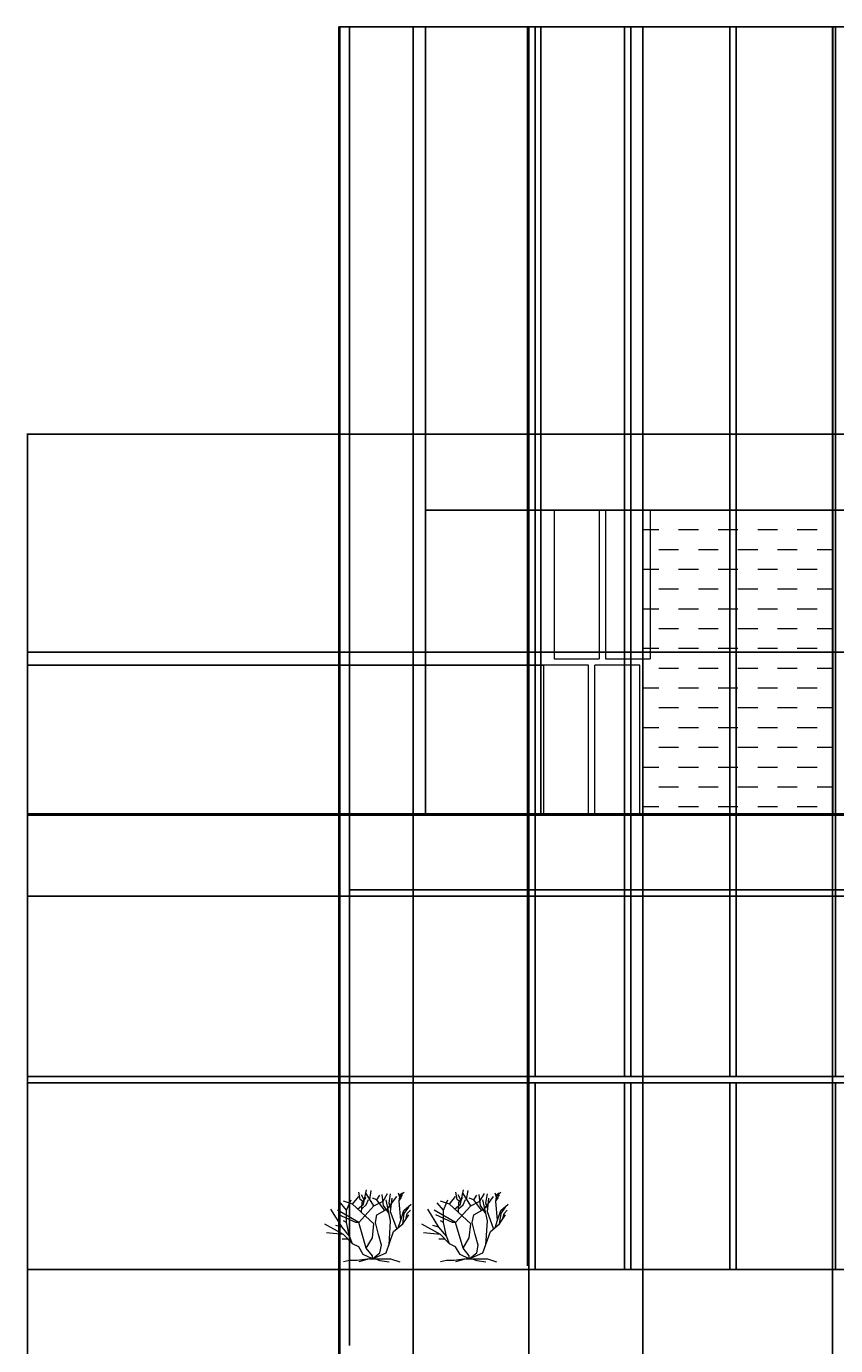
# Model space of a CAD drawing. Units: inches. Extents: x 250 to 1217, y -42 to 832.
# Tile 3 of 7: x 250 to 506, y 415 to 832. Entities that reach past the tile are written whole.
import ezdxf

# ---------------------------------------------------------------- set-up
doc = ezdxf.new("R2010")
doc.units = ezdxf.units.IN
doc.header["$MEASUREMENT"] = 0
for name, color, linetype, lineweight in [('A-ANNO-DIMS', 2, 'Continuous', 18), ('A-ELEV', 7, 'Continuous', 25), ('A-ELEV-PATT', 8, 'Continuous', 13), ('A-GLAZ', 4, 'Continuous', 18), ('L-PLNT', 3, 'Continuous', 13)]:
    doc.layers.add(name, color=color, linetype=linetype, lineweight=lineweight)
doc.styles.get("Standard").update_dxf_attribs({"font": 'arial.ttf'})
doc.dimstyles.get("Standard").update_dxf_attribs({"dimtxt": 0.18, "dimasz": 0.18, "dimexe": 0.18, "dimexo": 0.0625, "dimgap": 0.09, "dimtad": 0, "dimtih": 1, "dimtoh": 1, "dimdec": 4, "dimzin": 0, "dimdsep": 46, "dimtxsty": 'Standard', "dimcen": 0.09, "dimadec": 0, "dimazin": 0, "dimtfac": 1, "dimtdec": 4, "dimtofl": 0, "dimtmove": 0, "dimatfit": 3, "dimfxl": 1, "dimtolj": 1, "dimtzin": 0, "dimarcsym": 0})

# ---------------------------------------------------------------- blocks, each defined once
blk = doc.blocks.new('*U2')
for p, q in [((-12.471, 19.775), (-12.898, 22.044)), ((-11.28, 19.619), (-12.104, 21.184)), ((-11.433, 18.289), (-10.457, 22.749)), ((-8.16, 17.76), (-10.56, 21.6)), ((-9.48, 19.775), (-8.992, 22.592)), ((-7.2, 19.68), (-6.24, 21.12)), ((-5.086, 17.741), (-5.513, 21.34)), ((-5.28, 19.2), (-3.84, 21.6)), ((-3.377, 18.602), (-2.888, 21.575)), ((-0.508, 21.888), (-0.081, 20.558)), ((-0.203, 19.149), (0.102, 21.34)), ((-0.02, 20.01), (0.896, 21.105)), ((0.041, 20.714), (1.384, 22.044)), ((0.102, 21.34), (0.835, 21.888)), ((-16.8, 16.32), (-18.72, 18.72)), ((-14.88, 18.24), (-17.76, 19.2)), ((-16.8, 16.32), (-15.36, 19.68)), ((-14.88, 18.24), (-12.96, 20.64)), ((-8.16, 12), (-14.88, 18.24)), ((-13.325, 16.724), (-11.433, 18.289)), ((-12.96, 12.48), (-8.16, 17.76)), ((-11.677, 19.071), (-12.471, 19.775)), ((-12.043, 15.628), (-11.921, 18.836)), ((-11.982, 16.802), (-10.579, 18.054)), ((-11.921, 18.836), (-10.64, 20.401)), ((-10.579, 18.054), (-9.846, 19.697)), ((-7.2, 19.68), (-8.64, 20.16)), ((-8.16, 17.76), (-5.28, 19.2)), ((-4.8, 16.32), (-7.2, 19.68)), ((-7.2, 14.88), (-3.84, 16.8)), ((-3.377, 15.315), (-5.086, 17.819)), ((-2.88, 12.96), (-4.32, 19.68)), ((-3.84, 16.8), (-0.96, 20.64)), ((-2.766, 16.802), (-3.377, 18.602)), ((-2.88, 15.84), (-2.4, 20.16)), ((0.346, 13.203), (-0.203, 19.149)), ((-0.142, 19.384), (0.59, 20.401)), ((1.323, 16.254), (3.642, 18.289)), ((1.44, 15.36), (2.88, 17.28)), ((-18.24, 11.04), (-21.755, 16.655)), ((-12.96, 12.48), (-19.68, 16.32)), ((-13.92, 12.48), (-19.2, 14.88)), ((-16.8, 12.48), (-17.76, 12.96)), ((-16.8, 12.48), (-16.8, 16.32)), ((-7.68, 12.48), (-7.2, 14.88)), ((-3.36, 5.28), (-2.88, 12.96)), ((-0.96, 10.56), (-2.88, 15.84)), ((-0.48, 10.8), (0.346, 13.203)), ((0.346, 13.203), (1.323, 16.254)), ((0.96, 12), (1.44, 15.36)), ((0.96, 12), (2.88, 14.88)), ((1.92, 13.44), (2.4, 15.36)), ((2.4, 15.36), (3.36, 16.32)), ((-17.76, 8.64), (-23.663, 11.961)), ((-17.76, 8.64), (-23.128, 9.222)), ((-18.24, 11.04), (-20.16, 11.52)), ((-15.84, 8.16), (-18.24, 11.04)), ((-14.88, 5.76), (-17.76, 8.64)), ((-15.84, 8.16), (-16.8, 12.48)), ((-12.96, 12.48), (-13.92, 12.48)), ((-10.56, 4.32), (-12.96, 12.48)), ((-8.64, 7.68), (-8.16, 12)), ((-6.72, 8.64), (-7.68, 12.48)), ((-5.76, 5.28), (-6.72, 8.64)), ((-4.32, 2.88), (-1.92, 9.6)), ((-1.92, 9.6), (0.96, 12)), ((-16.32, 7.2), (-18.24, 7.2)), ((-14.88, 5.76), (-15.84, 8.16)), ((-12.96, 4.8), (-14.88, 5.76)), ((-11.52, 2.4), (-12.96, 4.8)), ((-10.56, 4.32), (-8.64, 7.68)), ((-8.64, 1.92), (-10.56, 4.32)), ((-6.24, 2.88), (-5.76, 5.28)), ((-15.84, 0.48), (-17.76, 0)), ((-13.44, 0.48), (-15.84, 0.48)), ((-9.6, 0.96), (-13.44, 0.48)), ((-9.6, 0.96), (-12.96, 0)), ((-8.64, 0.96), (-11.52, 2.4)), ((-9.6, 0.96), (-7.68, 0.96)), ((-8.64, 0.96), (-4.32, 2.88)), ((-8.64, 0.96), (-6.24, 2.88)), ((-8.64, 0.96), (-8.64, 1.92)), ((-8.64, 0.96), (-2.88, 0.96)), ((-7.68, 0.96), (-6.24, 0.48)), ((-6.24, 0.48), (-3.36, 0)), ((-2.88, 0.96), (0, 0))]:
    blk.add_line(p, q)
blk = doc.blocks.new('WIN-PANEL-NARROW')
for p, q in [((0, 47), (0, 0)), ((14.16, 47), (14.16, 0)), ((0, 0), (14.16, 0))]:
    blk.add_line(p, q)
blk = doc.blocks.new('*D8')
at = {"layer": 'A-ANNO-DIMS', "color": 0, "lineweight": -2, "transparency": 16777216}
for p, q in [((352.34, 702.99), (352.34, 831.77)), ((352.52, 831.59), (491.1, 831.59)), ((630.6, 831.59), (492.03, 831.59)), ((630.78, 702.99), (630.78, 831.77))]:
    blk.add_line(p, q, dxfattribs=at)
at = {"layer": 'A-ANNO-DIMS', "color": 0, "transparency": 16777216}
for points in [[(352.52, 831.62), (352.52, 831.56), (352.34, 831.59)], [(630.6, 831.62), (630.6, 831.56), (630.78, 831.59)]]:
    blk.add_solid(points, dxfattribs=at)
at = {"layer": 'Defpoints', "color": 0, "transparency": 16777216}
for p in [(630.78, 831.59), (352.34, 702.93), (630.78, 702.93)]:
    blk.add_point(p, dxfattribs=at)
at = {"layer": 'A-ANNO-DIMS', "color": 0, "transparency": 16777216, "insert": (491.56, 831.59), "char_height": 0.18, "attachment_point": 5}
blk.add_mtext('\\A1;278.44', dxfattribs=at)
blk = doc.blocks.new('*D11')
at = {"layer": 'A-ANNO-DIMS', "color": 0, "lineweight": -2, "transparency": 16777216}
for p, q in [((352.28, 702.93), (250.36, 702.93)), ((250.54, 702.75), (250.54, 390.68)), ((250.54, 78.24), (250.54, 390.31)), ((347.84, 78.06), (250.36, 78.06))]:
    blk.add_line(p, q, dxfattribs=at)
at = {"layer": 'A-ANNO-DIMS', "color": 0, "transparency": 16777216}
for points in [[(250.51, 702.75), (250.57, 702.75), (250.54, 702.93)], [(250.51, 78.24), (250.57, 78.24), (250.54, 78.06)]]:
    blk.add_solid(points, dxfattribs=at)
at = {"layer": 'Defpoints', "color": 0, "transparency": 16777216}
for p in [(250.54, 702.93), (352.34, 702.93), (347.9, 78.06)]:
    blk.add_point(p, dxfattribs=at)
at = {"layer": 'A-ANNO-DIMS', "color": 0, "transparency": 16777216, "insert": (250.54, 390.49), "char_height": 0.18, "attachment_point": 5}
blk.add_mtext('\\A1;624.9', dxfattribs=at)
blk = doc.blocks.new('*D22')
at = {"layer": 'A-ANNO-DIMS', "color": 0, "lineweight": -2, "transparency": 16777216}
for p, q in [((349.2, 175.91), (349.2, 831.77)), ((349.38, 831.59), (378.7, 831.59)), ((408.8, 831.59), (379.49, 831.59)), ((408.98, 174.99), (408.98, 831.77))]:
    blk.add_line(p, q, dxfattribs=at)
at = {"layer": 'A-ANNO-DIMS', "color": 0, "transparency": 16777216}
for points in [[(349.38, 831.62), (349.38, 831.56), (349.2, 831.59)], [(408.8, 831.62), (408.8, 831.56), (408.98, 831.59)]]:
    blk.add_solid(points, dxfattribs=at)
at = {"layer": 'Defpoints', "color": 0, "transparency": 16777216}
for p in [(408.98, 831.59), (349.2, 175.84), (408.98, 174.93)]:
    blk.add_point(p, dxfattribs=at)
at = {"layer": 'A-ANNO-DIMS', "color": 0, "transparency": 16777216, "insert": (379.09, 831.59), "char_height": 0.18, "attachment_point": 5}
blk.add_mtext('\\A1;59.78', dxfattribs=at)
blk = doc.blocks.new('*D23')
at = {"layer": 'A-ANNO-DIMS', "color": 0, "lineweight": -2, "transparency": 16777216}
for p, q in [((408.98, 174.99), (408.98, 831.77)), ((409.16, 831.59), (426.76, 831.59)), ((444.8, 831.59), (427.2, 831.59)), ((444.98, 174.99), (444.98, 831.77))]:
    blk.add_line(p, q, dxfattribs=at)
at = {"layer": 'A-ANNO-DIMS', "color": 0, "transparency": 16777216}
for points in [[(409.16, 831.62), (409.16, 831.56), (408.98, 831.59)], [(444.8, 831.62), (444.8, 831.56), (444.98, 831.59)]]:
    blk.add_solid(points, dxfattribs=at)
at = {"layer": 'Defpoints', "color": 0, "transparency": 16777216}
for p in [(444.98, 831.59), (408.98, 174.93), (444.98, 174.93)]:
    blk.add_point(p, dxfattribs=at)
at = {"layer": 'A-ANNO-DIMS', "color": 0, "transparency": 16777216, "insert": (426.98, 831.59), "char_height": 0.18, "attachment_point": 5}
blk.add_mtext('\\A1;36', dxfattribs=at)
blk = doc.blocks.new('*D24')
at = {"layer": 'A-ANNO-DIMS', "color": 0, "lineweight": -2, "transparency": 16777216}
for p, q in [((444.98, 174.99), (444.98, 831.77)), ((445.16, 831.59), (474.76, 831.59)), ((504.8, 831.59), (475.2, 831.59)), ((504.98, 174.99), (504.98, 831.77))]:
    blk.add_line(p, q, dxfattribs=at)
at = {"layer": 'A-ANNO-DIMS', "color": 0, "transparency": 16777216}
for points in [[(445.16, 831.62), (445.16, 831.56), (444.98, 831.59)], [(504.8, 831.62), (504.8, 831.56), (504.98, 831.59)]]:
    blk.add_solid(points, dxfattribs=at)
at = {"layer": 'Defpoints', "color": 0, "transparency": 16777216}
for p in [(504.98, 831.59), (444.98, 174.93), (504.98, 174.93)]:
    blk.add_point(p, dxfattribs=at)
at = {"layer": 'A-ANNO-DIMS', "color": 0, "transparency": 16777216, "insert": (474.98, 831.59), "char_height": 0.18, "attachment_point": 5}
blk.add_mtext('\\A1;60', dxfattribs=at)
blk = doc.blocks.new('*D25')
at = {"layer": 'A-ANNO-DIMS', "color": 0, "lineweight": -2, "transparency": 16777216}
for p, q in [((504.98, 174.99), (504.98, 831.77)), ((505.16, 831.59), (522.76, 831.59)), ((540.8, 831.59), (523.2, 831.59)), ((540.98, 174.99), (540.98, 831.77))]:
    blk.add_line(p, q, dxfattribs=at)
at = {"layer": 'A-ANNO-DIMS', "color": 0, "transparency": 16777216}
for points in [[(505.16, 831.62), (505.16, 831.56), (504.98, 831.59)], [(540.8, 831.62), (540.8, 831.56), (540.98, 831.59)]]:
    blk.add_solid(points, dxfattribs=at)
at = {"layer": 'Defpoints', "color": 0, "transparency": 16777216}
for p in [(540.98, 831.59), (504.98, 174.93), (540.98, 174.93)]:
    blk.add_point(p, dxfattribs=at)
at = {"layer": 'A-ANNO-DIMS', "color": 0, "transparency": 16777216, "insert": (522.98, 831.59), "char_height": 0.18, "attachment_point": 5}
blk.add_mtext('\\A1;36', dxfattribs=at)
blk = doc.blocks.new('*D38')
at = {"layer": 'A-ANNO-DIMS', "color": 0, "lineweight": -2, "transparency": 16777216}
for p, q in [((413.675954, 629.927068), (250.356906, 629.927068)), ((250.536906, 629.747068), (250.536906, 606.607068)), ((250.536906, 583.107068), (250.536906, 606.247068)), ((412.675954, 582.927068), (250.356906, 582.927068))]:
    blk.add_line(p, q, dxfattribs=at)
at = {"layer": 'A-ANNO-DIMS', "color": 0, "transparency": 16777216}
for points in [[(250.506906, 629.747068), (250.566906, 629.747068), (250.536906, 629.927068)], [(250.506906, 583.107068), (250.566906, 583.107068), (250.536906, 582.927068)]]:
    blk.add_solid(points, dxfattribs=at)
at = {"layer": 'Defpoints', "color": 0, "transparency": 16777216}
for p in [(250.536906, 629.927068), (413.738454, 629.927068), (412.738454, 582.927068)]:
    blk.add_point(p, dxfattribs=at)
at = {"layer": 'A-ANNO-DIMS', "color": 0, "transparency": 16777216, "insert": (250.536906, 606.427068), "char_height": 0.18, "attachment_point": 5}
blk.add_mtext('\\A1;47', dxfattribs=at)
blk = doc.blocks.new('*D39')
at = {"layer": 'A-ANNO-DIMS', "color": 0, "lineweight": -2, "transparency": 16777216}
for p, q in [((352.34, 558.99), (352.34, 831.77)), ((352.52, 831.59), (364.12, 831.59)), ((376.16, 831.59), (364.56, 831.59)), ((376.34, 582.99), (376.34, 831.77))]:
    blk.add_line(p, q, dxfattribs=at)
at = {"layer": 'A-ANNO-DIMS', "color": 0, "transparency": 16777216}
for points in [[(352.52, 831.62), (352.52, 831.56), (352.34, 831.59)], [(376.16, 831.62), (376.16, 831.56), (376.34, 831.59)]]:
    blk.add_solid(points, dxfattribs=at)
at = {"layer": 'Defpoints', "color": 0, "transparency": 16777216}
for p in [(352.34, 831.59), (376.34, 582.93), (352.34, 558.93)]:
    blk.add_point(p, dxfattribs=at)
at = {"layer": 'A-ANNO-DIMS', "color": 0, "transparency": 16777216, "insert": (364.34, 831.59), "char_height": 0.18, "attachment_point": 5}
blk.add_mtext('\\A1;24', dxfattribs=at)
blk = doc.blocks.new('*D40')
at = {"layer": 'A-ANNO-DIMS', "color": 0, "lineweight": -2, "transparency": 16777216}
for p, q in [((376.34, 678.99), (376.34, 831.77)), ((376.52, 831.59), (394.08, 831.59)), ((412.56, 831.59), (395, 831.59)), ((412.74, 678.99), (412.74, 831.77))]:
    blk.add_line(p, q, dxfattribs=at)
at = {"layer": 'A-ANNO-DIMS', "color": 0, "transparency": 16777216}
for points in [[(376.52, 831.62), (376.52, 831.56), (376.34, 831.59)], [(412.56, 831.62), (412.56, 831.56), (412.74, 831.59)]]:
    blk.add_solid(points, dxfattribs=at)
at = {"layer": 'Defpoints', "color": 0, "transparency": 16777216}
for p in [(412.74, 831.59), (376.34, 678.93), (412.74, 678.93)]:
    blk.add_point(p, dxfattribs=at)
at = {"layer": 'A-ANNO-DIMS', "color": 0, "transparency": 16777216, "insert": (394.54, 831.59), "char_height": 0.18, "attachment_point": 5}
blk.add_mtext('\\A1;36.396', dxfattribs=at)
blk = doc.blocks.new('*D41')
at = {"layer": 'A-ANNO-DIMS', "color": 0, "lineweight": -2, "transparency": 16777216}
for p, q in [((412.74, 678.99), (412.74, 831.77)), ((412.92, 831.59), (428.44, 831.59)), ((444.88, 831.59), (429.37, 831.59)), ((445.06, 678.99), (445.06, 831.77))]:
    blk.add_line(p, q, dxfattribs=at)
at = {"layer": 'A-ANNO-DIMS', "color": 0, "transparency": 16777216}
for points in [[(412.92, 831.62), (412.92, 831.56), (412.74, 831.59)], [(444.88, 831.62), (444.88, 831.56), (445.06, 831.59)]]:
    blk.add_solid(points, dxfattribs=at)
at = {"layer": 'Defpoints', "color": 0, "transparency": 16777216}
for p in [(445.06, 831.59), (412.74, 678.93), (445.06, 678.93)]:
    blk.add_point(p, dxfattribs=at)
at = {"layer": 'A-ANNO-DIMS', "color": 0, "transparency": 16777216, "insert": (428.9, 831.59), "char_height": 0.18, "attachment_point": 5}
blk.add_mtext('\\A1;32.326', dxfattribs=at)
blk = doc.blocks.new('*D42')
at = {"layer": 'A-ANNO-DIMS', "color": 0, "lineweight": -2, "transparency": 16777216}
for p, q in [((445.06, 678.99), (445.06, 831.77)), ((445.24, 831.59), (474.85, 831.59)), ((504.88, 831.59), (475.28, 831.59)), ((505.06, 678.99), (505.06, 831.77))]:
    blk.add_line(p, q, dxfattribs=at)
at = {"layer": 'A-ANNO-DIMS', "color": 0, "transparency": 16777216}
for points in [[(445.24, 831.62), (445.24, 831.56), (445.06, 831.59)], [(504.88, 831.62), (504.88, 831.56), (505.06, 831.59)]]:
    blk.add_solid(points, dxfattribs=at)
at = {"layer": 'Defpoints', "color": 0, "transparency": 16777216}
for p in [(505.06, 831.59), (445.06, 678.93), (505.06, 678.93)]:
    blk.add_point(p, dxfattribs=at)
at = {"layer": 'A-ANNO-DIMS', "color": 0, "transparency": 16777216, "insert": (475.06, 831.59), "char_height": 0.18, "attachment_point": 5}
blk.add_mtext('\\A1;60', dxfattribs=at)
blk = doc.blocks.new('*D43')
at = {"layer": 'A-ANNO-DIMS', "color": 0, "lineweight": -2, "transparency": 16777216}
for p, q in [((505.06, 678.99), (505.06, 831.77)), ((505.24, 831.59), (512.61, 831.59)), ((520.89, 831.59), (513.52, 831.59)), ((521.07, 678.99), (521.07, 831.77))]:
    blk.add_line(p, q, dxfattribs=at)
at = {"layer": 'A-ANNO-DIMS', "color": 0, "transparency": 16777216}
for points in [[(505.24, 831.62), (505.24, 831.56), (505.06, 831.59)], [(520.89, 831.62), (520.89, 831.56), (521.07, 831.59)]]:
    blk.add_solid(points, dxfattribs=at)
at = {"layer": 'Defpoints', "color": 0, "transparency": 16777216}
for p in [(521.07, 831.59), (505.06, 678.93), (521.07, 678.93)]:
    blk.add_point(p, dxfattribs=at)
at = {"layer": 'A-ANNO-DIMS', "color": 0, "transparency": 16777216, "insert": (513.07, 831.59), "char_height": 0.18, "attachment_point": 5}
blk.add_mtext('\\A1;16.002', dxfattribs=at)
blk = doc.blocks.new('*D49')
at = {"layer": 'A-ANNO-DIMS', "color": 0, "lineweight": -2, "transparency": 16777216}
for p, q in [((348.98, 318.99), (348.98, 831.77)), ((349.16, 831.59), (489.48, 831.59)), ((630.6, 831.59), (490.28, 831.59)), ((630.78, 318.99), (630.78, 831.77))]:
    blk.add_line(p, q, dxfattribs=at)
at = {"layer": 'A-ANNO-DIMS', "color": 0, "transparency": 16777216}
for points in [[(349.16, 831.62), (349.16, 831.56), (348.98, 831.59)], [(630.6, 831.62), (630.6, 831.56), (630.78, 831.59)]]:
    blk.add_solid(points, dxfattribs=at)
at = {"layer": 'Defpoints', "color": 0, "transparency": 16777216}
for p in [(630.78, 831.59), (348.98, 318.93), (630.78, 318.93)]:
    blk.add_point(p, dxfattribs=at)
at = {"layer": 'A-ANNO-DIMS', "color": 0, "transparency": 16777216, "insert": (489.88, 831.59), "char_height": 0.18, "attachment_point": 5}
blk.add_mtext('\\A1;281.8', dxfattribs=at)
blk = doc.blocks.new('*D51')
at = {"layer": 'A-ANNO-DIMS', "color": 0, "lineweight": -2, "transparency": 16777216}
for p, q in [((348.98, 198.99), (348.98, 831.77)), ((349.16, 831.59), (360.27, 831.59)), ((372.3, 831.59), (361.2, 831.59)), ((372.48, 199.88), (372.48, 831.77))]:
    blk.add_line(p, q, dxfattribs=at)
at = {"layer": 'A-ANNO-DIMS', "color": 0, "transparency": 16777216}
for points in [[(349.16, 831.62), (349.16, 831.56), (348.98, 831.59)], [(372.3, 831.62), (372.3, 831.56), (372.48, 831.59)]]:
    blk.add_solid(points, dxfattribs=at)
at = {"layer": 'Defpoints', "color": 0, "transparency": 16777216}
for p in [(372.48, 831.59), (348.98, 198.93), (372.48, 199.81)]:
    blk.add_point(p, dxfattribs=at)
at = {"layer": 'A-ANNO-DIMS', "color": 0, "transparency": 16777216, "insert": (360.73, 831.59), "char_height": 0.18, "attachment_point": 5}
blk.add_mtext('\\A1;23.496', dxfattribs=at)
blk = doc.blocks.new('*D53')
at = {"layer": 'A-ANNO-DIMS', "color": 0, "lineweight": -2, "transparency": 16777216}
for p, q in [((352.34, 438.99), (352.34, 831.77)), ((352.52, 831.59), (380.04, 831.59)), ((408.34, 831.59), (380.83, 831.59)), ((408.52, 440.1), (408.52, 831.77))]:
    blk.add_line(p, q, dxfattribs=at)
at = {"layer": 'A-ANNO-DIMS', "color": 0, "transparency": 16777216}
for points in [[(352.52, 831.62), (352.52, 831.56), (352.34, 831.59)], [(408.34, 831.62), (408.34, 831.56), (408.52, 831.59)]]:
    blk.add_solid(points, dxfattribs=at)
at = {"layer": 'Defpoints', "color": 0, "transparency": 16777216}
for p in [(408.52, 831.59), (352.34, 438.93), (408.52, 440.03)]:
    blk.add_point(p, dxfattribs=at)
at = {"layer": 'A-ANNO-DIMS', "color": 0, "transparency": 16777216, "insert": (380.43, 831.59), "char_height": 0.18, "attachment_point": 5}
blk.add_mtext('\\A1;56.18', dxfattribs=at)
blk = doc.blocks.new('*D54')
at = {"layer": 'A-ANNO-DIMS', "color": 0, "lineweight": -2, "transparency": 16777216}
for p, q in [((408.52, 440.1), (408.52, 831.77)), ((408.7, 831.59), (474.4, 831.59)), ((541, 831.59), (475.31, 831.59)), ((541.18, 438.99), (541.18, 831.77))]:
    blk.add_line(p, q, dxfattribs=at)
at = {"layer": 'A-ANNO-DIMS', "color": 0, "transparency": 16777216}
for points in [[(408.7, 831.62), (408.7, 831.56), (408.52, 831.59)], [(541, 831.62), (541, 831.56), (541.18, 831.59)]]:
    blk.add_solid(points, dxfattribs=at)
at = {"layer": 'Defpoints', "color": 0, "transparency": 16777216}
for p in [(541.18, 831.59), (408.52, 440.03), (541.18, 438.93)]:
    blk.add_point(p, dxfattribs=at)
at = {"layer": 'A-ANNO-DIMS', "color": 0, "transparency": 16777216, "insert": (474.85, 831.59), "char_height": 0.18, "attachment_point": 5}
blk.add_mtext('\\A1;132.66', dxfattribs=at)
blk = doc.blocks.new('*D78')
at = {"layer": 'A-ANNO-DIMS', "color": 0, "lineweight": -2, "transparency": 16777216}
for p, q in [((410.98, 556.99), (410.98, 831.77)), ((411.16, 831.59), (424.74, 831.59)), ((439.1, 831.59), (425.53, 831.59)), ((439.28, 556.99), (439.28, 831.77))]:
    blk.add_line(p, q, dxfattribs=at)
at = {"layer": 'A-ANNO-DIMS', "color": 0, "transparency": 16777216}
for points in [[(411.16, 831.62), (411.16, 831.56), (410.98, 831.59)], [(439.1, 831.62), (439.1, 831.56), (439.28, 831.59)]]:
    blk.add_solid(points, dxfattribs=at)
at = {"layer": 'Defpoints', "color": 0, "transparency": 16777216}
for p in [(439.28, 831.59), (410.98, 556.93), (439.28, 556.93)]:
    blk.add_point(p, dxfattribs=at)
at = {"layer": 'A-ANNO-DIMS', "color": 0, "transparency": 16777216, "insert": (425.13, 831.59), "char_height": 0.18, "attachment_point": 5}
blk.add_mtext('\\A1;28.30', dxfattribs=at)
blk = doc.blocks.new('*D79')
at = {"layer": 'A-ANNO-DIMS', "color": 0, "lineweight": -2, "transparency": 16777216}
for p, q in [((439.28, 556.99), (439.28, 831.77)), ((439.46, 831.59), (439.96, 831.59)), ((441.1, 831.59), (440.61, 831.59)), ((441.28, 556.99), (441.28, 831.77))]:
    blk.add_line(p, q, dxfattribs=at)
at = {"layer": 'A-ANNO-DIMS', "color": 0, "transparency": 16777216}
for points in [[(439.46, 831.62), (439.46, 831.56), (439.28, 831.59)], [(441.1, 831.62), (441.1, 831.56), (441.28, 831.59)]]:
    blk.add_solid(points, dxfattribs=at)
at = {"layer": 'Defpoints', "color": 0, "transparency": 16777216}
for p in [(441.28, 831.59), (439.28, 556.93), (441.28, 556.93)]:
    blk.add_point(p, dxfattribs=at)
at = {"layer": 'A-ANNO-DIMS', "color": 0, "transparency": 16777216, "insert": (440.28, 831.59), "char_height": 0.18, "attachment_point": 5}
blk.add_mtext('\\A1;2.00', dxfattribs=at)
blk = doc.blocks.new('*D80')
at = {"layer": 'A-ANNO-DIMS', "color": 0, "lineweight": -2, "transparency": 16777216}
for p, q in [((441.28, 556.99), (441.28, 831.77)), ((441.46, 831.59), (456.54, 831.59)), ((472.4, 831.59), (457.32, 831.59)), ((472.58, 556.99), (472.58, 831.77))]:
    blk.add_line(p, q, dxfattribs=at)
at = {"layer": 'A-ANNO-DIMS', "color": 0, "transparency": 16777216}
for points in [[(441.46, 831.62), (441.46, 831.56), (441.28, 831.59)], [(472.4, 831.62), (472.4, 831.56), (472.58, 831.59)]]:
    blk.add_solid(points, dxfattribs=at)
at = {"layer": 'Defpoints', "color": 0, "transparency": 16777216}
for p in [(472.58, 831.59), (441.28, 556.93), (472.58, 556.93)]:
    blk.add_point(p, dxfattribs=at)
at = {"layer": 'A-ANNO-DIMS', "color": 0, "transparency": 16777216, "insert": (456.93, 831.59), "char_height": 0.18, "attachment_point": 5}
blk.add_mtext('\\A1;31.30', dxfattribs=at)
blk = doc.blocks.new('*D81')
at = {"layer": 'A-ANNO-DIMS', "color": 0, "lineweight": -2, "transparency": 16777216}
for p, q in [((474.58, 556.99), (474.58, 831.77)), ((474.76, 831.59), (489.84, 831.59)), ((505.7, 831.59), (490.62, 831.59)), ((505.88, 556.99), (505.88, 831.77))]:
    blk.add_line(p, q, dxfattribs=at)
at = {"layer": 'A-ANNO-DIMS', "color": 0, "transparency": 16777216}
for points in [[(474.76, 831.62), (474.76, 831.56), (474.58, 831.59)], [(505.7, 831.62), (505.7, 831.56), (505.88, 831.59)]]:
    blk.add_solid(points, dxfattribs=at)
at = {"layer": 'Defpoints', "color": 0, "transparency": 16777216}
for p in [(505.88, 831.59), (474.58, 556.93), (505.88, 556.93)]:
    blk.add_point(p, dxfattribs=at)
at = {"layer": 'A-ANNO-DIMS', "color": 0, "transparency": 16777216, "insert": (490.23, 831.59), "char_height": 0.18, "attachment_point": 5}
blk.add_mtext('\\A1;31.30', dxfattribs=at)
blk = doc.blocks.new('*D83')
at = {"layer": 'A-ANNO-DIMS', "color": 0, "lineweight": -2, "transparency": 16777216}
for p, q in [((539.12, 497.99), (250.36, 497.99)), ((250.54, 497.81), (250.54, 468.64)), ((250.54, 439.11), (250.54, 468.28)), ((539.12, 438.93), (250.36, 438.93))]:
    blk.add_line(p, q, dxfattribs=at)
at = {"layer": 'A-ANNO-DIMS', "color": 0, "transparency": 16777216}
for points in [[(250.51, 497.81), (250.57, 497.81), (250.54, 497.99)], [(250.51, 439.11), (250.57, 439.11), (250.54, 438.93)]]:
    blk.add_solid(points, dxfattribs=at)
at = {"layer": 'Defpoints', "color": 0, "transparency": 16777216}
for p in [(250.54, 497.99), (539.18, 497.99), (539.18, 438.93)]:
    blk.add_point(p, dxfattribs=at)
at = {"layer": 'A-ANNO-DIMS', "color": 0, "transparency": 16777216, "insert": (250.54, 468.46), "char_height": 0.18, "attachment_point": 5}
blk.add_mtext('\\A1;59.06', dxfattribs=at)
blk = doc.blocks.new('*D84')
at = {"layer": 'A-ANNO-DIMS', "color": 0, "lineweight": -2, "transparency": 16777216}
for p, q in [((539.12, 499.99), (250.36, 499.99)), ((539.12, 497.99), (250.36, 497.99)), ((250.54, 499.81), (250.54, 499.17)), ((250.54, 498.17), (250.54, 498.81))]:
    blk.add_line(p, q, dxfattribs=at)
at = {"layer": 'A-ANNO-DIMS', "color": 0, "transparency": 16777216}
for points in [[(250.51, 499.81), (250.57, 499.81), (250.54, 499.99)], [(250.51, 498.17), (250.57, 498.17), (250.54, 497.99)]]:
    blk.add_solid(points, dxfattribs=at)
at = {"layer": 'Defpoints', "color": 0, "transparency": 16777216}
for p in [(250.54, 499.99), (539.18, 499.99), (539.18, 497.99)]:
    blk.add_point(p, dxfattribs=at)
at = {"layer": 'A-ANNO-DIMS', "color": 0, "transparency": 16777216, "insert": (250.54, 498.99), "char_height": 0.18, "attachment_point": 5}
blk.add_mtext('\\A1;2.00', dxfattribs=at)
blk = doc.blocks.new('*D85')
at = {"layer": 'A-ANNO-DIMS', "color": 0, "lineweight": -2, "transparency": 16777216}
for p, q in [((539.12, 556.93), (250.36, 556.93)), ((250.54, 556.75), (250.54, 528.64)), ((250.54, 500.17), (250.54, 528.28)), ((539.12, 499.99), (250.36, 499.99))]:
    blk.add_line(p, q, dxfattribs=at)
at = {"layer": 'A-ANNO-DIMS', "color": 0, "transparency": 16777216}
for points in [[(250.51, 556.75), (250.57, 556.75), (250.54, 556.93)], [(250.51, 500.17), (250.57, 500.17), (250.54, 499.99)]]:
    blk.add_solid(points, dxfattribs=at)
at = {"layer": 'Defpoints', "color": 0, "transparency": 16777216}
for p in [(250.54, 556.93), (539.18, 556.93), (539.18, 499.99)]:
    blk.add_point(p, dxfattribs=at)
at = {"layer": 'A-ANNO-DIMS', "color": 0, "transparency": 16777216, "insert": (250.54, 528.46), "char_height": 0.18, "attachment_point": 5}
blk.add_mtext('\\A1;56.94', dxfattribs=at)
blk = doc.blocks.new('*D86')
at = {"layer": 'A-ANNO-DIMS', "color": 0, "lineweight": -2, "transparency": 16777216}
for p, q in [((410.92, 556.93), (250.36, 556.93)), ((250.54, 556.75), (250.54, 498.11)), ((250.54, 439.11), (250.54, 497.75)), ((410.92, 438.93), (250.36, 438.93))]:
    blk.add_line(p, q, dxfattribs=at)
at = {"layer": 'A-ANNO-DIMS', "color": 0, "transparency": 16777216}
for points in [[(250.51, 556.75), (250.57, 556.75), (250.54, 556.93)], [(250.51, 439.11), (250.57, 439.11), (250.54, 438.93)]]:
    blk.add_solid(points, dxfattribs=at)
at = {"layer": 'Defpoints', "color": 0, "transparency": 16777216}
for p in [(250.54, 556.93), (410.98, 556.93), (410.98, 438.93)]:
    blk.add_point(p, dxfattribs=at)
at = {"layer": 'A-ANNO-DIMS', "color": 0, "transparency": 16777216, "insert": (250.54, 497.93), "char_height": 0.18, "attachment_point": 5}
blk.add_mtext('\\A1;118.00', dxfattribs=at)
blk = doc.blocks.new('*D94')
at = {"layer": 'A-ANNO-DIMS', "color": 0, "lineweight": -2, "transparency": 16777216}
for p, q in [((601.99, 633.99), (250.36, 633.99)), ((250.54, 633.81), (250.54, 608.47)), ((250.54, 582.76), (250.54, 608.1)), ((597.96, 582.58), (250.36, 582.58))]:
    blk.add_line(p, q, dxfattribs=at)
at = {"layer": 'A-ANNO-DIMS', "color": 0, "transparency": 16777216}
for points in [[(250.51, 633.81), (250.57, 633.81), (250.54, 633.99)], [(250.51, 582.76), (250.57, 582.76), (250.54, 582.58)]]:
    blk.add_solid(points, dxfattribs=at)
at = {"layer": 'Defpoints', "color": 0, "transparency": 16777216}
for p in [(250.54, 633.99), (602.05, 633.99), (598.03, 582.58)]:
    blk.add_point(p, dxfattribs=at)
at = {"layer": 'A-ANNO-DIMS', "color": 0, "transparency": 16777216, "insert": (250.54, 608.29), "char_height": 0.18, "attachment_point": 5}
blk.add_mtext('\\A1;51.41', dxfattribs=at)

msp = doc.modelspace()

# ---------------------------------------------------------------- hatches: boundary and pattern name
at = {"layer": 'A-ELEV-PATT'}
h = msp.add_hatch(dxfattribs=at)
h.set_pattern_fill('DASH', color=256, scale=50)
h.set_pattern_definition([(0, (0.0823, 504), (6.25, 6.25), [6.25, -6.25])])
h.paths.add_polyline_path([(505.0649, 678.9271), (445.0649, 678.9271), (445.0649, 582.9271), (505.0649, 582.9271)])

# ---------------------------------------------------------------- linework, layer by layer
at = {"layer": 'A-ELEV'}
for p, q in [((412.7385, 678.9271), (412.7385, 582.9271)), ((412.7385, 678.9271), (412.7385, 582.9271)), ((412.7385, 678.9271), (412.7385, 582.9271)), ((412.7385, 678.9271), (412.7385, 582.9271)), ((445.0649, 678.9271), (445.0649, 582.9271)), ((445.0649, 678.9271), (445.0649, 582.9271)), ((445.0649, 678.9271), (445.0649, 582.9271)), ((445.0649, 678.9271), (445.0649, 582.9271)), ((505.0649, 678.9271), (505.0649, 582.9271)), ((505.0649, 678.9271), (505.0649, 582.9271)), ((505.0649, 678.9271), (505.0649, 582.9271)), ((505.0649, 678.9271), (505.0649, 582.9271)), ((505.0649, 678.9271), (505.0649, 582.9271)), ((352.3429, 558.9271), (352.3429, 582.9271)), ((376.3429, 582.9271), (630.7779, 582.9271)), ((376.3429, 582.9271), (630.7779, 582.9271)), ((352.3429, 558.9271), (630.7779, 558.9271)), ((408.9826, 438.9271), (408.9826, 558.9271)), ((408.9826, 558.9271), (541.1795, 558.9271)), ((410.9826, 556.9271), (539.1795, 556.9271)), ((410.9826, 499.991), (410.9826, 556.9271)), ((439.2815, 499.991), (439.2815, 556.9271)), ((441.2815, 499.991), (441.2815, 556.9271)), ((472.5809, 499.991), (472.5809, 556.9271)), ((474.5809, 499.991), (474.5809, 556.9271)), ((505.8802, 499.991), (505.8802, 556.9271)), ((410.9826, 499.991), (439.2815, 499.991)), ((410.9826, 438.9271), (410.9826, 497.991)), ((410.9826, 497.991), (439.2815, 497.991)), ((439.2815, 438.9271), (439.2815, 497.991)), ((441.2815, 499.991), (472.5809, 499.991)), ((441.2815, 438.9271), (441.2815, 497.991)), ((441.2815, 497.991), (472.5809, 497.991)), ((472.5809, 438.9271), (472.5809, 497.991)), ((474.5809, 499.991), (505.8802, 499.991)), ((474.5809, 438.9271), (474.5809, 497.991)), ((474.5809, 497.991), (505.8802, 497.991)), ((505.8802, 438.9271), (505.8802, 497.991)), ((352.3429, 438.9271), (630.7779, 438.9271)), ((352.3429, 414.9271), (352.3429, 438.9271))]:
    msp.add_line(p, q, dxfattribs=at)
for points in [[(952.2329, 582.9271), (952.2329, 702.9271), (352.3429, 702.9271), (352.3429, 582.9271)], [(630.7779, 678.9271), (376.3429, 678.9271), (376.3429, 582.9271)]]:
    msp.add_lwpolyline(points, dxfattribs=at)

# ---------------------------------------------------------------- block references
at = {"layer": 'A-GLAZ'}
for p in [(417.0163, 631.927), (433.1796, 631.927)]:
    msp.add_blockref('WIN-PANEL-NARROW', p, dxfattribs=at)
at = {"layer": 'A-GLAZ', "rotation": 180}
for p in [(427.9018, 629.9271), (444.065, 629.9271)]:
    msp.add_blockref('WIN-PANEL-NARROW', p, dxfattribs=at)
at = {"layer": 'L-PLNT'}
for p in [(368.1829, 441.3562), (398.7837, 441.3562)]:
    msp.add_blockref('*U2', p, dxfattribs=at)

# ---------------------------------------------------------------- dimensions: what is measured, and where the dimension line sits
at = {"layer": 'A-ANNO-DIMS'}
for base, p1, p2, override, picture, middle in [((630.7779, 831.5941), (348.9826, 318.9271), (630.7779, 318.9271), {"dimdec": 1, "dimlfac": 1, "dimrnd": 0, "dimzin": 0, "dimdsep": 46, "dimlunit": 2}, '*D49', (489.8803, 831.5941)), ((372.4789, 831.5941), (348.9826, 198.9271), (372.4789, 199.8131), {"dimdec": 3, "dimlfac": 1, "dimrnd": 0, "dimzin": 0, "dimdsep": 46, "dimlunit": 2}, '*D51', (360.7307, 831.5941)), ((408.9826, 831.5941), (349.204, 175.8442), (408.9826, 174.9271), {"dimdec": 2, "dimlfac": 1, "dimrnd": 0, "dimzin": 0, "dimdsep": 46, "dimlunit": 2}, '*D22', (379.0933, 831.5941)), ((630.77793, 831.59407), (352.34291, 702.92707), (630.77793, 702.92707), {"dimdec": 2, "dimlfac": 1, "dimrnd": 0, "dimzin": 0, "dimdsep": 46, "dimlunit": 2}, '*D8', (491.56042, 831.59407)), ((352.3429, 831.5941), (376.3429, 582.9271), (352.3429, 558.9271), {"dimdec": 0, "dimlfac": 1, "dimrnd": 0, "dimzin": 0, "dimdsep": 46, "dimlunit": 2}, '*D39', (364.3429, 831.5941)), ((408.5234, 831.5941), (352.3429, 438.9271), (408.5234, 440.0339), {"dimdec": 2, "dimlfac": 1, "dimrnd": 0, "dimzin": 0, "dimdsep": 46, "dimlunit": 2}, '*D53', (380.4332, 831.5941)), ((412.7385, 831.5941), (376.3429, 678.9271), (412.7385, 678.9271), {"dimdec": 3, "dimlfac": 1, "dimrnd": 0, "dimzin": 0, "dimdsep": 46, "dimlunit": 2}, '*D40', (394.5407, 831.5941)), ((541.1795, 831.5941), (408.5234, 440.0339), (541.1795, 438.9271), {"dimdec": 2, "dimlfac": 1, "dimrnd": 0, "dimzin": 0, "dimdsep": 46, "dimlunit": 2}, '*D54', (474.8515, 831.5941)), ((444.9826, 831.5941), (408.9826, 174.9271), (444.9826, 174.9271), {"dimdec": 0, "dimlfac": 1, "dimrnd": 0, "dimzin": 0, "dimdsep": 46, "dimlunit": 2}, '*D23', (426.9826, 831.5941)), ((439.2815, 831.5941), (410.9826, 556.9271), (439.2815, 556.9271), {"dimdec": 2, "dimlfac": 1, "dimrnd": 0, "dimzin": 0, "dimdsep": 46, "dimlunit": 2}, '*D78', (425.1321, 831.5941)), ((445.0649, 831.5941), (412.7385, 678.9271), (445.0649, 678.9271), {"dimdec": 3, "dimlfac": 1, "dimrnd": 0, "dimzin": 0, "dimdsep": 46, "dimlunit": 2}, '*D41', (428.9017, 831.5941)), ((441.2815, 831.5941), (439.2815, 556.9271), (441.2815, 556.9271), {"dimdec": 2, "dimlfac": 1, "dimrnd": 0, "dimzin": 0, "dimdsep": 46, "dimlunit": 2}, '*D79', (440.2815, 831.5941)), ((472.5809, 831.5941), (441.2815, 556.9271), (472.5809, 556.9271), {"dimdec": 2, "dimlfac": 1, "dimrnd": 0, "dimzin": 0, "dimdsep": 46, "dimlunit": 2}, '*D80', (456.9312, 831.5941)), ((504.9826, 831.5941), (444.9826, 174.9271), (504.9826, 174.9271), {"dimdec": 0, "dimlfac": 1, "dimrnd": 0, "dimzin": 0, "dimdsep": 46, "dimlunit": 2}, '*D24', (474.9826, 831.5941)), ((505.0649, 831.5941), (445.0649, 678.9271), (505.0649, 678.9271), {"dimdec": 0, "dimlfac": 1, "dimrnd": 0, "dimzin": 0, "dimdsep": 46, "dimlunit": 2}, '*D42', (475.0649, 831.5941)), ((505.8802, 831.5941), (474.5809, 556.9271), (505.8802, 556.9271), {"dimdec": 2, "dimlfac": 1, "dimrnd": 0, "dimzin": 0, "dimdsep": 46, "dimlunit": 2}, '*D81', (490.2305, 831.5941)), ((540.9826, 831.5941), (504.9826, 174.9271), (540.9826, 174.9271), {"dimdec": 0, "dimlfac": 1, "dimrnd": 0, "dimzin": 0, "dimdsep": 46, "dimlunit": 2}, '*D25', (522.9826, 831.5941)), ((521.0669, 831.5941), (505.0649, 678.9271), (521.0669, 678.9271), {"dimdec": 3, "dimlfac": 1, "dimrnd": 0, "dimzin": 0, "dimdsep": 46, "dimlunit": 2}, '*D43', (513.0659, 831.5941))]:
    dim = msp.add_linear_dim(base=base, p1=p1, p2=p2, dimstyle='Standard', override=override, dxfattribs=at)
    dim.commit()
    dim.dimension.update_dxf_attribs({"geometry": picture, "text_midpoint": middle})
for base, p1, p2, override, picture, middle in [((250.5369, 702.9271), (347.8976, 78.0612), (352.3429, 702.9271), {"dimdec": 1, "dimlfac": 1, "dimrnd": 0, "dimzin": 0, "dimdsep": 46, "dimlunit": 2}, '*D11', (250.5369, 390.4941)), ((250.5369, 633.9889), (598.0256, 582.5825), (602.051, 633.9889), {"dimdec": 2, "dimlfac": 1, "dimrnd": 0, "dimzin": 0, "dimdsep": 46, "dimlunit": 2}, '*D94', (250.5369, 608.2857)), ((250.5369, 629.9271), (412.7385, 582.9271), (413.7385, 629.9271), {"dimdec": 0, "dimlfac": 1, "dimrnd": 0, "dimzin": 0, "dimdsep": 46, "dimlunit": 2}, '*D38', (250.5369, 606.4271)), ((250.5369, 556.9271), (410.9826, 438.9271), (410.9826, 556.9271), {"dimdec": 2, "dimlfac": 1, "dimrnd": 0, "dimzin": 0, "dimdsep": 46, "dimlunit": 2}, '*D86', (250.5369, 497.9271)), ((250.5369, 556.9271), (539.1795, 499.991), (539.1795, 556.9271), {"dimdec": 2, "dimlfac": 1, "dimrnd": 0, "dimzin": 0, "dimdsep": 46, "dimlunit": 2}, '*D85', (250.5369, 528.459)), ((250.5369, 497.991), (539.1795, 438.9271), (539.1795, 497.991), {"dimdec": 2, "dimlfac": 1, "dimrnd": 0, "dimzin": 0, "dimdsep": 46, "dimlunit": 2}, '*D83', (250.5369, 468.459)), ((250.5369, 499.991), (539.1795, 497.991), (539.1795, 499.991), {"dimdec": 2, "dimlfac": 1, "dimrnd": 0, "dimzin": 0, "dimdsep": 46, "dimlunit": 2}, '*D84', (250.5369, 498.991))]:
    dim = msp.add_linear_dim(base=base, p1=p1, p2=p2, angle=90, dimstyle='Standard', override=override, dxfattribs=at)
    dim.commit()
    dim.dimension.update_dxf_attribs({"geometry": picture, "text_midpoint": middle})

doc.saveas('drawing.dxf')
